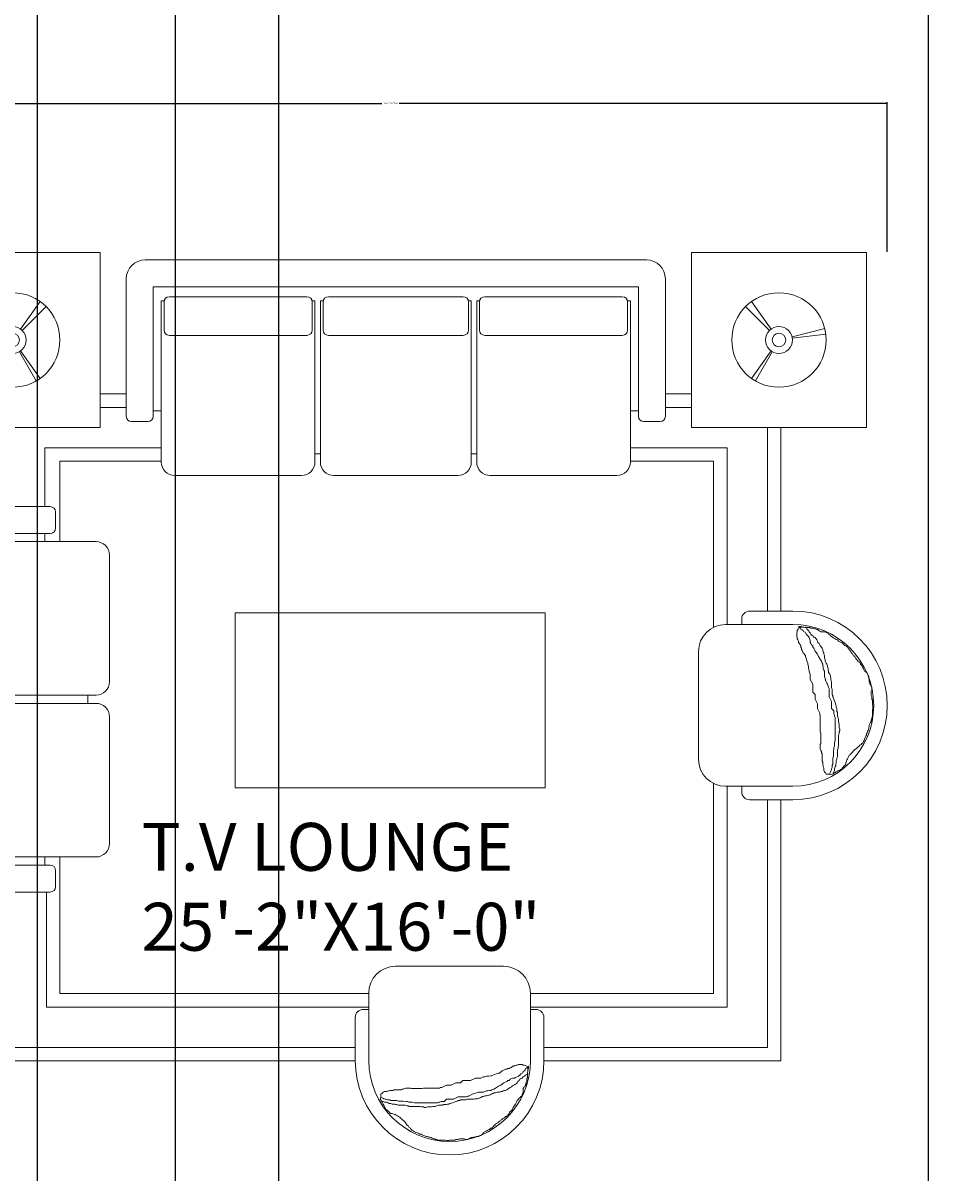
# Model space of a CAD drawing. Units: inches. Extents: x 2447 to 3157, y 2799 to 3988.
# Tile 6 of 9: x 2810 to 2947, y 3441 to 3609. Entities that reach past the tile are written whole.
import ezdxf

# ---------------------------------------------------------------- set-up
doc = ezdxf.new("R2010")
doc.units = ezdxf.units.IN
for name, color, linetype, lineweight in [('A-ANNO-DIMS', 2, 'Continuous', 18), ('A-AREA-IDEN', 7, 'Continuous', 25), ('A-FURN', 8, 'Continuous', 18)]:
    doc.layers.add(name, color=color, linetype=linetype, lineweight=lineweight)
doc.styles.get("Standard").update_dxf_attribs({"font": 'arial.ttf'})
doc.dimstyles.get("Standard").update_dxf_attribs({"dimtxt": 0.18, "dimasz": 0.18, "dimexe": 0.18, "dimexo": 0.0625, "dimgap": 0.09, "dimtad": 0, "dimtih": 1, "dimtoh": 1, "dimdec": 4, "dimzin": 0, "dimdsep": 46, "dimtxsty": 'Standard', "dimcen": 0.09, "dimadec": 0, "dimazin": 0, "dimtfac": 1, "dimtdec": 4, "dimtofl": 0, "dimtmove": 0, "dimatfit": 3, "dimfxl": 1, "dimtolj": 1, "dimtzin": 0, "dimarcsym": 0})

# ---------------------------------------------------------------- blocks, each defined once
blk = doc.blocks.new('A$C78064EA7')
for p, q in [((932.1, 3320.6), (2792.1, 3320.6)), ((862.1, 2740.6), (862.1, 3250.6)), ((2862.1, 3250.6), (2862.1, 2740.6)), ((962.1, 3220.6), (962.1, 2740.6)), ((2762.1, 3220.6), (962.1, 3220.6)), ((2762.1, 2740.6), (2762.1, 3220.6)), ((469.8, 3064.3), (542.4, 3166)), ((992.1, 3168.5), (1002.1, 3168.5)), ((992.1, 2570.6), (992.1, 3168.5)), ((1002.1, 3060.6), (1002.1, 3164.3)), ((1022.1, 3184.3), (1532.1, 3184.3)), ((1551.6, 3168.5), (1562.1, 3168.5)), ((1552.1, 3060.6), (1552.1, 3164.3)), ((1562.1, 2570.6), (1562.1, 3168.5)), ((1582.1, 3168.5), (1592.5, 3168.5)), ((1582.1, 2570.6), (1582.1, 3168.5)), ((1592.1, 3060.6), (1592.1, 3164.3)), ((1612.1, 3184.3), (2112.1, 3184.3)), ((2131.6, 3168.5), (2142.1, 3168.5)), ((2132.1, 3060.6), (2132.1, 3164.3)), ((2142.1, 2570.6), (2142.1, 3168.5)), ((2162.1, 3168.5), (2172.5, 3168.5)), ((2162.1, 2570.6), (2162.1, 3168.5)), ((2172.1, 3060.6), (2172.1, 3164.3)), ((2192.1, 3184.3), (2702.1, 3184.3)), ((2721.6, 3168.5), (2732.1, 3168.5)), ((2722.1, 3060.6), (2722.1, 3164.3)), ((2732.1, 3168.5), (2732.1, 2570.6)), ((3254.4, 3064.3), (3181.7, 3166)), ((476.1, 3059), (564.4, 3147.3)), ((3248.1, 3059), (3159.7, 3147.3)), ((391.1, 3029.8), (267.1, 3045.3)), ((392.2, 3035.7), (270.9, 3066)), ((1022.1, 3040.6), (1532.1, 3040.6)), ((1612.1, 3040.6), (2112.1, 3040.6)), ((2192.1, 3040.6), (2702.1, 3040.6)), ((3331.9, 3035.7), (3453.2, 3066)), ((3333, 3029.8), (3457.1, 3045.3)), ((465.5, 2980.2), (527.5, 2871.7)), ((469.8, 2982.9), (542.4, 2881.2)), ((3254.4, 2982.9), (3181.7, 2881.2)), ((3258.6, 2980.2), (3196.6, 2871.7)), ((862.1, 2823.6), (765.7, 2823.6)), ((2958.4, 2823.6), (2862.1, 2823.6)), ((862.1, 2773.6), (765.7, 2773.6)), ((2958.4, 2773.6), (2862.1, 2773.6)), ((962.1, 2760.6), (992.1, 2760.6)), ((2732.1, 2760.6), (2762.1, 2760.6)), ((365.7, 2698.6), (365.7, 2405.5)), ((415.7, 2698.6), (415.7, 2405.5)), ((942.1, 2720.6), (882.1, 2720.6)), ((2842.1, 2720.6), (2782.1, 2720.6)), ((3240.7, 2017.9), (3240.7, 2698.6)), ((3290.7, 2017.9), (3290.7, 2698.6)), ((992.1, 2623.6), (560, 2623.6)), ((560, 2405.5), (560, 2623.6)), ((992.1, 2573.6), (615.7, 2573.6)), ((615.7, 2573.6), (615.7, 2275.5)), ((1562.1, 2600.6), (1582.1, 2600.6)), ((2142.1, 2600.6), (2162.1, 2600.6)), ((1042.1, 2520.6), (1512.1, 2520.6)), ((1632.1, 2520.6), (2092.1, 2520.6)), ((2212.1, 2520.6), (2682.1, 2520.6)), ((70, 2405.5), (580, 2405.5)), ((600, 2385.5), (600, 2325.5)), ((0, 1045.5), (0, 2335.5)), ((580, 2305.5), (100, 2305.5)), ((100, 2305.5), (100, 1075.5)), ((560, 2275.5), (560, 2305.5)), ((152.1, 2275.5), (750, 2275.5)), ((152.1, 2265.1), (152.1, 2275.5)), ((260, 2265.5), (156.3, 2265.5)), ((136.3, 1735.5), (136.3, 2245.5)), ((280, 1735.5), (280, 2245.5)), ((800, 1755.5), (800, 2225.5)), ((3335.1, 2017.9), (3175.1, 2017.9)), ((3335.1, 1967.9), (3085.1, 1967.9)), ((3145.1, 1987.9), (3145.1, 1967.9)), ((3351.6, 1941.1), (3349.3, 1936.8)), ((3349.3, 1936.8), (3349.3, 1923.5)), ((3349.3, 1923.5), (3351.6, 1919.2)), ((3353.6, 1950), (3351.6, 1945.4)), ((3351.6, 1945.4), (3351.6, 1941.1)), ((3358.2, 1958.7), (3353.6, 1950)), ((3358.2, 1961), (3355.9, 1961)), ((3362.5, 1958.7), (3358.2, 1961)), ((3362.5, 1961), (3358.2, 1958.7)), ((3358.2, 1958.7), (3362.5, 1954.4)), ((3366.8, 1961), (3362.5, 1961)), ((3375.5, 1958.7), (3362.5, 1958.7)), ((3362.5, 1954.4), (3364.5, 1950)), ((3364.5, 1950), (3369.1, 1947.7)), ((3369.1, 1947.7), (3373.5, 1945.4)), ((3373.5, 1945.4), (3375.5, 1941.1)), ((3380.1, 1956.4), (3375.5, 1958.7)), ((3375.5, 1941.1), (3380.1, 1939.1)), ((3397.4, 1956.4), (3380.1, 1956.4)), ((3380.1, 1939.1), (3384.4, 1932.4)), ((3384.4, 1958.7), (3382.1, 1958.7)), ((3386.4, 1954.4), (3384.4, 1958.7)), ((3384.4, 1932.4), (3388.7, 1928.1)), ((3388.7, 1950), (3386.4, 1954.4)), ((3393.1, 1945.4), (3388.7, 1950)), ((3388.7, 1928.1), (3393.1, 1923.5)), ((3395.4, 1941.1), (3393.1, 1945.4)), ((3393.1, 1923.5), (3395.4, 1919.2)), ((3399.7, 1936.8), (3395.4, 1941.1)), ((3402, 1954.4), (3397.4, 1956.4)), ((3402, 1932.4), (3399.7, 1936.8)), ((3410.6, 1954.4), (3402, 1954.4)), ((3404, 1928.1), (3402, 1932.4)), ((3408.6, 1925.8), (3404, 1928.1)), ((3412.9, 1921.5), (3408.6, 1925.8)), ((3415, 1952.1), (3410.6, 1954.4)), ((3417.3, 1919.2), (3412.9, 1921.5)), ((3419.6, 1952.1), (3415, 1952.1)), ((3423.9, 1950), (3419.6, 1952.1)), ((3428.2, 1950), (3423.9, 1950)), ((3430.5, 1945.4), (3428.2, 1950)), ((3434.8, 1943.4), (3430.5, 1945.4)), ((3439.2, 1941.1), (3434.8, 1943.4)), ((3452.4, 1941.1), (3439.2, 1941.1)), ((3456.7, 1939.1), (3452.4, 1941.1)), ((3461.1, 1936.8), (3456.7, 1939.1)), ((3465.4, 1936.8), (3461.1, 1936.8)), ((3467.7, 1932.4), (3465.4, 1936.8)), ((3472, 1930.1), (3467.7, 1932.4)), ((3474.3, 1925.8), (3472, 1930.1)), ((3478.7, 1923.5), (3474.3, 1925.8)), ((3483, 1919.2), (3478.7, 1923.5)), ((3351.6, 1919.2), (3351.6, 1914.9)), ((3351.6, 1914.9), (3353.6, 1910.5)), ((3353.6, 1910.5), (3355.9, 1906.2)), ((3355.9, 1906.2), (3355.9, 1901.6)), ((3355.9, 1901.6), (3360.2, 1897.3)), ((3360.2, 1897.3), (3362.5, 1892.9)), ((3362.5, 1892.9), (3364.5, 1888.6)), ((3364.5, 1888.6), (3364.5, 1884.3)), ((3364.5, 1884.3), (3366.8, 1879.7)), ((3366.8, 1879.7), (3366.8, 1875.3)), ((3395.4, 1919.2), (3397.4, 1912.5)), ((3397.4, 1912.5), (3399.7, 1908.2)), ((3399.7, 1908.2), (3399.7, 1901.6)), ((3399.7, 1901.6), (3402, 1897.3)), ((3402, 1897.3), (3404, 1892.9)), ((3404, 1892.9), (3408.6, 1888.6)), ((3408.6, 1888.6), (3408.6, 1884.3)), ((3408.6, 1884.3), (3412.9, 1879.7)), ((3412.9, 1879.7), (3417.3, 1869)), ((3421.6, 1914.9), (3417.3, 1919.2)), ((3423.9, 1910.5), (3421.6, 1914.9)), ((3425.9, 1906.2), (3423.9, 1910.5)), ((3428.2, 1901.6), (3425.9, 1906.2)), ((3432.5, 1897.3), (3428.2, 1901.6)), ((3434.8, 1892.9), (3432.5, 1897.3)), ((3436.9, 1888.6), (3434.8, 1892.9)), ((3441.5, 1884.3), (3436.9, 1888.6)), ((3443.5, 1879.7), (3441.5, 1884.3)), ((3445.8, 1875.3), (3443.5, 1879.7)), ((3487.3, 1917.2), (3483, 1919.2)), ((3491.6, 1914.9), (3487.3, 1917.2)), ((3496.2, 1912.5), (3491.6, 1914.9)), ((3500.6, 1910.5), (3496.2, 1912.5)), ((3504.9, 1906.2), (3500.6, 1910.5)), ((3509.2, 1903.9), (3504.9, 1906.2)), ((3513.8, 1901.6), (3509.2, 1903.9)), ((3518.1, 1899.6), (3513.8, 1901.6)), ((3522.5, 1895.2), (3518.1, 1899.6)), ((3526.8, 1890.6), (3522.5, 1895.2)), ((3531.1, 1888.6), (3526.8, 1890.6)), ((3535.7, 1886.3), (3531.1, 1888.6)), ((3537.7, 1882), (3535.7, 1886.3)), ((3542.1, 1879.7), (3537.7, 1882)), ((3542.1, 1875.3), (3542.1, 1879.7)), ((2985.1, 1867.9), (2985.1, 1467.9)), ((3366.8, 1875.3), (3369.1, 1871)), ((3369.1, 1871), (3373.5, 1862.3)), ((3373.5, 1862.3), (3382.1, 1853.4)), ((3382.1, 1853.4), (3382.1, 1849.1)), ((3382.1, 1849.1), (3384.4, 1842.4)), ((3384.4, 1842.4), (3386.4, 1833.8)), ((3417.3, 1869), (3425.9, 1858)), ((3425.9, 1858), (3430.5, 1849.1)), ((3430.5, 1849.1), (3434.8, 1842.4)), ((3434.8, 1842.4), (3436.9, 1838.1)), ((3436.9, 1838.1), (3441.5, 1831.5)), ((3445.8, 1871), (3445.8, 1875.3)), ((3447.8, 1866.7), (3445.8, 1871)), ((3450.1, 1862.3), (3447.8, 1866.7)), ((3450.1, 1858), (3450.1, 1862.3)), ((3452.4, 1853.4), (3450.1, 1858)), ((3452.4, 1844.8), (3452.4, 1853.4)), ((3454.4, 1838.1), (3452.4, 1844.8)), ((3454.4, 1833.8), (3454.4, 1838.1)), ((3546.7, 1873.3), (3542.1, 1875.3)), ((3548.7, 1869), (3546.7, 1873.3)), ((3551, 1864.4), (3548.7, 1869)), ((3555.3, 1860), (3551, 1864.4)), ((3557.6, 1855.7), (3555.3, 1860)), ((3561.9, 1853.4), (3557.6, 1855.7)), ((3561.9, 1849.1), (3561.9, 1853.4)), ((3566.3, 1847.1), (3561.9, 1849.1)), ((3568.6, 1842.4), (3566.3, 1847.1)), ((3570.6, 1838.1), (3568.6, 1842.4)), ((3574.9, 1836.1), (3570.6, 1838.1)), ((3574.9, 1831.5), (3574.9, 1836.1)), ((3386.4, 1833.8), (3391, 1825.1)), ((3391, 1825.1), (3391, 1820.5)), ((3391, 1820.5), (3393.1, 1811.9)), ((3393.1, 1811.9), (3393.1, 1805.2)), ((3393.1, 1805.2), (3395.4, 1798.6)), ((3395.4, 1798.6), (3395.4, 1792.2)), ((3395.4, 1792.2), (3399.7, 1783.3)), ((3441.5, 1831.5), (3443.5, 1825.1)), ((3443.5, 1825.1), (3445.8, 1820.5)), ((3445.8, 1820.5), (3445.8, 1816.2)), ((3445.8, 1816.2), (3447.8, 1809.6)), ((3447.8, 1809.6), (3447.8, 1805.2)), ((3447.8, 1805.2), (3450.1, 1798.6)), ((3450.1, 1798.6), (3452.4, 1794.3)), ((3452.4, 1794.3), (3452.4, 1774.7)), ((3456.7, 1829.5), (3454.4, 1833.8)), ((3458.8, 1825.1), (3456.7, 1829.5)), ((3461.1, 1820.5), (3458.8, 1825.1)), ((3463.4, 1816.2), (3461.1, 1820.5)), ((3463.4, 1811.9), (3463.4, 1816.2)), ((3465.4, 1805.2), (3463.4, 1811.9)), ((3465.4, 1798.6), (3465.4, 1805.2)), ((3467.7, 1794.3), (3465.4, 1798.6)), ((3467.7, 1789.9), (3467.7, 1794.3)), ((3579.5, 1831.5), (3574.9, 1831.5)), ((3581.5, 1827.2), (3579.5, 1831.5)), ((3585.9, 1825.1), (3581.5, 1827.2)), ((3585.9, 1820.5), (3585.9, 1825.1)), ((3590.5, 1816.2), (3585.9, 1820.5)), ((3592.5, 1811.9), (3590.5, 1816.2)), ((3594.8, 1807.5), (3592.5, 1811.9)), ((3596.8, 1803.2), (3594.8, 1807.5)), ((3599.1, 1798.6), (3596.8, 1803.2)), ((3601.4, 1794.3), (3599.1, 1798.6)), ((3605.7, 1792.2), (3601.4, 1794.3)), ((3610.1, 1787.6), (3605.7, 1792.2)), ((3399.7, 1783.3), (3399.7, 1763.7)), ((3399.7, 1763.7), (3408.6, 1746.1)), ((3452.4, 1774.7), (3454.4, 1768)), ((3454.4, 1768), (3456.7, 1761.4)), ((3456.7, 1761.4), (3458.8, 1755)), ((3458.8, 1755), (3461.1, 1750.4)), ((3461.1, 1750.4), (3463.4, 1746.1)), ((3472, 1783.3), (3467.7, 1789.9)), ((3474.3, 1779), (3472, 1783.3)), ((3474.3, 1774.7), (3474.3, 1779)), ((3476.3, 1770.3), (3474.3, 1774.7)), ((3476.3, 1761.4), (3476.3, 1770.3)), ((3478.7, 1757.1), (3476.3, 1761.4)), ((3478.7, 1733.1), (3478.7, 1757.1)), ((3612.4, 1783.3), (3610.1, 1787.6)), ((3614.4, 1779), (3612.4, 1783.3)), ((3616.7, 1774.7), (3614.4, 1779)), ((3616.7, 1766), (3616.7, 1774.7)), ((3618.7, 1761.4), (3616.7, 1766)), ((3618.7, 1757.1), (3618.7, 1761.4)), ((3621, 1752.7), (3618.7, 1757.1)), ((3621, 1748.4), (3621, 1752.7)), ((152.1, 1705.5), (152.1, 1716)), ((260, 1715.5), (156.3, 1715.5)), ((3408.6, 1746.1), (3408.6, 1717.5)), ((3408.6, 1717.5), (3417.3, 1708.9)), ((3417.3, 1708.9), (3417.3, 1691.3)), ((3463.4, 1746.1), (3465.4, 1739.5)), ((3465.4, 1739.5), (3467.7, 1735.1)), ((3467.7, 1735.1), (3469.7, 1730.8)), ((3469.7, 1730.8), (3469.7, 1700.2)), ((3480.7, 1728.5), (3478.7, 1733.1)), ((3480.7, 1708.9), (3480.7, 1728.5)), ((3483, 1704.6), (3480.7, 1708.9)), ((3623.3, 1744.1), (3621, 1748.4)), ((3625.3, 1739.5), (3623.3, 1744.1)), ((3627.6, 1735.1), (3625.3, 1739.5)), ((3625.3, 1722.1), (3627.6, 1726.5)), ((3625.3, 1704.6), (3625.3, 1722.1)), ((3627.6, 1726.5), (3627.6, 1735.1)), ((750, 1705.5), (152.1, 1705.5)), ((750, 1675.5), (152.1, 1675.5)), ((152.1, 1665.1), (152.1, 1675.5)), ((260, 1665.5), (156.3, 1665.5)), ((720, 1685.5), (720, 1705.5)), ((720, 1675.5), (720, 1695.5)), ((3417.3, 1691.3), (3425.9, 1674)), ((3425.9, 1674), (3425.9, 1656.4)), ((3469.7, 1700.2), (3478.7, 1682.6)), ((3478.7, 1682.6), (3478.7, 1656.4)), ((3483, 1700.2), (3483, 1704.6)), ((3485.3, 1695.6), (3483, 1700.2)), ((3487.3, 1691.3), (3485.3, 1695.6)), ((3491.6, 1678.3), (3487.3, 1691.3)), ((3493.9, 1669.4), (3491.6, 1678.3)), ((3496.2, 1665), (3493.9, 1669.4)), ((3496.2, 1660.7), (3496.2, 1665)), ((3627.6, 1700.2), (3625.3, 1704.6)), ((3627.6, 1691.3), (3627.6, 1700.2)), ((3629.9, 1687), (3627.6, 1691.3)), ((3629.9, 1669.4), (3629.9, 1687)), ((3632, 1665), (3629.9, 1669.4)), ((3632, 1656.4), (3632, 1665)), ((136.3, 1135.5), (136.3, 1645.5)), ((280, 1135.5), (280, 1645.5)), ((800, 1155.5), (800, 1625.5)), ((3425.9, 1656.4), (3434.8, 1638.8)), ((3434.8, 1638.8), (3434.8, 1634.5)), ((3434.8, 1634.5), (3436.9, 1630.1)), ((3436.9, 1630.1), (3436.9, 1571)), ((3478.7, 1656.4), (3487.3, 1647.4)), ((3487.3, 1647.4), (3487.3, 1636.5)), ((3487.3, 1636.5), (3489.6, 1632.1)), ((3489.6, 1632.1), (3489.6, 1627.8)), ((3489.6, 1627.8), (3491.6, 1623.5)), ((3491.6, 1623.5), (3491.6, 1538.1)), ((3498.2, 1656.4), (3496.2, 1660.7)), ((3498.2, 1645.4), (3498.2, 1656.4)), ((3500.6, 1641.1), (3498.2, 1645.4)), ((3500.6, 1627.8), (3500.6, 1641.1)), ((3502.6, 1621.2), (3500.6, 1627.8)), ((3627.6, 1621.2), (3629.9, 1625.5)), ((3629.9, 1652), (3632, 1656.4)), ((3629.9, 1625.5), (3629.9, 1652)), ((3504.9, 1614.5), (3502.6, 1621.2)), ((3504.9, 1605.9), (3504.9, 1614.5)), ((3507.2, 1599.3), (3504.9, 1605.9)), ((3507.2, 1586.3), (3507.2, 1599.3)), ((3509.2, 1579.6), (3507.2, 1586.3)), ((3509.2, 1575.3), (3509.2, 1579.6)), ((3614.4, 1575.3), (3616.7, 1582)), ((3616.7, 1586.3), (3618.7, 1590.6)), ((3616.7, 1582), (3616.7, 1586.3)), ((3618.7, 1594.9), (3621, 1599.3)), ((3618.7, 1590.6), (3618.7, 1594.9)), ((3621, 1599.3), (3623.3, 1603.9)), ((3623.3, 1603.9), (3625.3, 1608.2)), ((3625.3, 1612.5), (3627.6, 1616.9)), ((3625.3, 1608.2), (3625.3, 1612.5)), ((3627.6, 1616.9), (3627.6, 1621.2)), ((3436.9, 1571), (3439.2, 1564.4)), ((3439.2, 1564.4), (3439.2, 1527.1)), ((3491.6, 1538.1), (3489.6, 1529.2)), ((3504.9, 1557.7), (3507.2, 1562)), ((3504.9, 1518.2), (3504.9, 1557.7)), ((3507.2, 1571), (3509.2, 1575.3)), ((3507.2, 1562), (3507.2, 1571)), ((3596.8, 1533.5), (3599.1, 1538.1)), ((3599.1, 1538.1), (3601.4, 1542.4)), ((3601.4, 1542.4), (3603.4, 1549.1)), ((3603.4, 1549.1), (3605.7, 1553.4)), ((3605.7, 1553.4), (3607.8, 1557.7)), ((3607.8, 1562), (3610.1, 1566.4)), ((3607.8, 1557.7), (3607.8, 1562)), ((3610.1, 1566.4), (3612.4, 1571)), ((3612.4, 1571), (3614.4, 1575.3)), ((3439.2, 1527.1), (3436.9, 1522.5)), ((3436.9, 1522.5), (3436.9, 1505.2)), ((3436.9, 1505.2), (3439.2, 1500.9)), ((3439.2, 1500.9), (3441.5, 1496.3)), ((3441.5, 1496.3), (3441.5, 1491.9)), ((3487.3, 1507.2), (3485.3, 1496.3)), ((3485.3, 1496.3), (3485.3, 1479)), ((3489.6, 1516.2), (3487.3, 1511.9)), ((3487.3, 1511.9), (3487.3, 1507.2)), ((3489.6, 1529.2), (3489.6, 1516.2)), ((3500.6, 1502.9), (3502.6, 1509.5)), ((3500.6, 1476.7), (3500.6, 1502.9)), ((3502.6, 1513.9), (3504.9, 1518.2)), ((3502.6, 1509.5), (3502.6, 1513.9)), ((3551, 1489.9), (3564, 1502.9)), ((3564, 1502.9), (3572.9, 1509.5)), ((3572.9, 1509.5), (3577.2, 1513.9)), ((3577.2, 1513.9), (3581.5, 1516.2)), ((3581.5, 1516.2), (3583.8, 1520.5)), ((3583.8, 1520.5), (3588.2, 1522.5)), ((3588.2, 1522.5), (3590.5, 1527.1)), ((3590.5, 1527.1), (3594.8, 1529.2)), ((3594.8, 1529.2), (3596.8, 1533.5)), ((3441.5, 1491.9), (3443.5, 1487.6)), ((3443.5, 1487.6), (3443.5, 1461.4)), ((3443.5, 1461.4), (3445.8, 1457)), ((3445.8, 1457), (3445.8, 1448.1)), ((3485.3, 1479), (3483, 1472.3)), ((3483, 1472.3), (3483, 1450.4)), ((3493.9, 1450.4), (3496.2, 1454.7)), ((3496.2, 1463.4), (3498.2, 1468)), ((3496.2, 1454.7), (3496.2, 1463.4)), ((3498.2, 1472.3), (3500.6, 1476.7)), ((3498.2, 1468), (3498.2, 1472.3)), ((3531.1, 1454.7), (3533.4, 1461.4)), ((3531.1, 1450.4), (3531.1, 1454.7)), ((3533.4, 1461.4), (3535.7, 1465.7)), ((3535.7, 1465.7), (3537.7, 1470)), ((3537.7, 1470), (3540, 1474.3)), ((3540, 1474.3), (3542.1, 1479)), ((3542.1, 1479), (3544.4, 1483.3)), ((3544.4, 1483.3), (3548.7, 1485.3)), ((3548.7, 1485.3), (3551, 1489.9)), ((3445.8, 1448.1), (3447.8, 1443.8)), ((3447.8, 1443.8), (3447.8, 1439.4)), ((3447.8, 1439.4), (3450.1, 1435.1)), ((3450.1, 1435.1), (3450.1, 1426.2)), ((3450.1, 1426.2), (3452.4, 1421.8)), ((3452.4, 1421.8), (3456.7, 1417.5)), ((3456.7, 1417.5), (3458.8, 1413.2)), ((3458.8, 1413.2), (3472, 1413.2)), ((3474.3, 1419.8), (3472, 1415.2)), ((3472, 1415.2), (3472, 1413.2)), ((3472, 1413.2), (3476.3, 1410.9)), ((3476.3, 1424.2), (3474.3, 1419.8)), ((3478.7, 1428.5), (3476.3, 1424.2)), ((3476.3, 1410.9), (3480.7, 1413.2)), ((3480.7, 1437.1), (3478.7, 1432.8)), ((3478.7, 1432.8), (3478.7, 1428.5)), ((3483, 1450.4), (3480.7, 1446.1)), ((3480.7, 1446.1), (3480.7, 1437.1)), ((3480.7, 1413.2), (3485.3, 1415.2)), ((3485.3, 1417.5), (3487.3, 1421.8)), ((3485.3, 1413.2), (3485.3, 1417.5)), ((3485.3, 1415.2), (3489.6, 1417.5)), ((3487.3, 1421.8), (3489.6, 1426.2)), ((3489.6, 1435.1), (3491.6, 1439.4)), ((3489.6, 1426.2), (3489.6, 1435.1)), ((3489.6, 1417.5), (3496.2, 1421.8)), ((3491.6, 1439.4), (3493.9, 1443.8)), ((3493.9, 1443.8), (3493.9, 1450.4)), ((3496.2, 1421.8), (3500.6, 1424.2)), ((3500.6, 1424.2), (3504.9, 1426.2)), ((3504.9, 1426.2), (3509.2, 1426.2)), ((3509.2, 1426.2), (3511.5, 1430.5)), ((3511.5, 1430.5), (3515.8, 1430.5)), ((3515.8, 1430.5), (3518.1, 1435.1)), ((3518.1, 1435.1), (3522.5, 1439.4)), ((3522.5, 1439.4), (3524.8, 1443.8)), ((3524.8, 1443.8), (3529.1, 1446.1)), ((3529.1, 1446.1), (3531.1, 1450.4)), ((3335.1, 1367.9), (3085.1, 1367.9)), ((3145.1, 1367.9), (3145.1, 1347.9)), ((3175.1, 1317.9), (3335.1, 1317.9)), ((152.1, 1105.5), (152.1, 1115.5)), ((260, 1115.5), (156.3, 1115.5)), ((100, 1075.5), (580, 1075.5)), ((750, 1105.5), (152.1, 1105.5)), ((560, 1075.5), (560, 1105.5)), ((600, 1055.5), (600, 995.5)), ((580, 975.5), (70, 975.5)), ((2261.5, 700), (1861.5, 700)), ((1761.5, 350), (1761.5, 600)), ((2361.5, 350), (2361.5, 600)), ((1761.5, 540), (1741.5, 540)), ((2381.5, 540), (2361.5, 540)), ((1711.5, 510), (1711.5, 350)), ((2411.5, 350), (2411.5, 510)), ((2236.1, 300.7), (2227.4, 298.6)), ((2242.7, 303), (2236.1, 300.7)), ((2247, 303), (2242.7, 303)), ((2256, 311.6), (2247, 303)), ((2264.6, 315.9), (2256, 311.6)), ((2269, 318.2), (2264.6, 315.9)), ((2273.3, 318.2), (2269, 318.2)), ((2277.9, 320.5), (2273.3, 318.2)), ((2282.2, 320.5), (2277.9, 320.5)), ((2286.6, 322.6), (2282.2, 320.5)), ((2290.9, 324.9), (2286.6, 322.6)), ((2295.2, 329.2), (2290.9, 324.9)), ((2299.8, 329.2), (2295.2, 329.2)), ((2304.2, 331.5), (2299.8, 329.2)), ((2308.5, 333.5), (2304.2, 331.5)), ((2312.8, 333.5), (2308.5, 333.5)), ((2317.1, 335.8), (2312.8, 333.5)), ((2330.4, 335.8), (2317.1, 335.8)), ((2326.1, 300.7), (2321.8, 296.3)), ((2332.7, 305), (2326.1, 300.7)), ((2334.7, 333.5), (2330.4, 335.8)), ((2334.7, 309.6), (2332.7, 305)), ((2339.1, 333.5), (2334.7, 333.5)), ((2339.1, 311.6), (2334.7, 309.6)), ((2343.7, 331.5), (2339.1, 333.5)), ((2341.4, 315.9), (2339.1, 311.6)), ((2343.7, 320.5), (2341.4, 315.9)), ((2352.3, 326.9), (2343.7, 331.5)), ((2348, 322.6), (2343.7, 320.5)), ((2352.3, 326.9), (2348, 322.6)), ((2348, 298.6), (2352.3, 300.7)), ((2350, 305), (2352.3, 309.6)), ((2350, 287.7), (2350, 305)), ((2352.3, 322.6), (2354.6, 326.9)), ((2354.6, 322.6), (2352.3, 326.9)), ((2352.3, 309.6), (2352.3, 322.6)), ((2352.3, 300.7), (2352.3, 303)), ((2354.6, 326.9), (2354.6, 329.2)), ((2354.6, 318.2), (2354.6, 322.6)), ((2050, 259.2), (2032.4, 250.2)), ((2067.6, 259.2), (2050, 259.2)), ((2084.9, 267.8), (2067.6, 259.2)), ((2102.5, 267.8), (2084.9, 267.8)), ((2111.2, 276.5), (2102.5, 267.8)), ((2139.7, 276.5), (2111.2, 276.5)), ((2157.3, 285.4), (2139.7, 276.5)), ((2176.9, 285.4), (2157.3, 285.4)), ((2185.9, 289.7), (2176.9, 285.4)), ((2192.2, 289.7), (2185.9, 289.7)), ((2198.9, 292), (2192.2, 289.7)), ((2205.5, 292), (2198.9, 292)), ((2214.2, 294), (2205.5, 292)), ((2218.8, 294), (2214.2, 294)), ((2227.4, 298.6), (2218.8, 294)), ((2251.7, 259.2), (2242.7, 254.6)), ((2262.6, 267.8), (2251.7, 259.2)), ((2273.3, 272.1), (2262.6, 267.8)), ((2277.9, 276.5), (2273.3, 272.1)), ((2282.2, 276.5), (2277.9, 276.5)), ((2286.6, 281.1), (2282.2, 276.5)), ((2290.9, 283.1), (2286.6, 281.1)), ((2295.2, 285.4), (2290.9, 283.1)), ((2290.9, 252.5), (2295.2, 256.9)), ((2301.9, 285.4), (2295.2, 285.4)), ((2295.2, 256.9), (2299.8, 259.2)), ((2299.8, 259.2), (2304.2, 261.2)), ((2306.2, 287.7), (2301.9, 285.4)), ((2304.2, 261.2), (2308.5, 263.5)), ((2312.8, 289.7), (2306.2, 287.7)), ((2308.5, 263.5), (2312.8, 267.8)), ((2317.1, 292), (2312.8, 289.7)), ((2312.8, 267.8), (2315.1, 272.1)), ((2315.1, 272.1), (2319.5, 276.5)), ((2321.8, 296.3), (2317.1, 292)), ((2319.5, 276.5), (2321.8, 281.1)), ((2321.8, 281.1), (2326.1, 283.1)), ((2326.1, 283.1), (2330.4, 285.4)), ((2330.4, 285.4), (2334.7, 289.7)), ((2334.7, 289.7), (2339.1, 292)), ((2339.1, 292), (2343.7, 296.3)), ((2339.1, 254.6), (2343.7, 256.9)), ((2343.7, 296.3), (2348, 298.6)), ((2343.7, 261.2), (2345.7, 265.5)), ((2343.7, 256.9), (2343.7, 261.2)), ((2345.7, 270.1), (2348, 274.4)), ((2345.7, 265.5), (2345.7, 270.1)), ((2348, 283.1), (2350, 287.7)), ((2348, 274.4), (2348, 283.1)), ((1811.2, 228.3), (1806.8, 226.3)), ((1806.8, 226.3), (1806.8, 213.1)), ((1815.5, 232.7), (1811.2, 228.3)), ((1819.8, 235), (1815.5, 232.7)), ((1828.8, 235), (1819.8, 235)), ((1833.1, 237.3), (1828.8, 235)), ((1837.4, 237.3), (1833.1, 237.3)), ((1841.7, 239.3), (1837.4, 237.3)), ((1850.7, 239.3), (1841.7, 239.3)), ((1855, 241.6), (1850.7, 239.3)), ((1881.3, 241.6), (1855, 241.6)), ((1885.6, 243.6), (1881.3, 241.6)), ((1889.9, 243.6), (1885.6, 243.6)), ((1894.5, 245.9), (1889.9, 243.6)), ((1898.9, 248.2), (1894.5, 245.9)), ((1916.2, 248.2), (1898.9, 248.2)), ((1920.8, 245.9), (1916.2, 248.2)), ((1958, 245.9), (1920.8, 245.9)), ((1964.6, 248.2), (1958, 245.9)), ((2023.8, 248.2), (1964.6, 248.2)), ((2028.1, 250.2), (2023.8, 248.2)), ((2032.4, 250.2), (2028.1, 250.2)), ((2093.9, 215.4), (2076.3, 206.4)), ((2124.4, 215.4), (2093.9, 215.4)), ((2128.8, 217.4), (2124.4, 215.4)), ((2133.1, 219.7), (2128.8, 217.4)), ((2139.7, 221.7), (2133.1, 219.7)), ((2144.1, 224), (2139.7, 221.7)), ((2148.7, 226.3), (2144.1, 224)), ((2155, 228.3), (2148.7, 226.3)), ((2161.7, 230.6), (2155, 228.3)), ((2168.3, 232.7), (2161.7, 230.6)), ((2187.9, 232.7), (2168.3, 232.7)), ((2176.9, 213.1), (2183.6, 217.4)), ((2183.6, 217.4), (2187.9, 217.4)), ((2192.2, 235), (2187.9, 232.7)), ((2187.9, 217.4), (2192.2, 219.7)), ((2198.9, 237.3), (2192.2, 235)), ((2192.2, 219.7), (2198.9, 219.7)), ((2203.2, 237.3), (2198.9, 237.3)), ((2198.9, 219.7), (2205.5, 221.7)), ((2209.8, 239.3), (2203.2, 237.3)), ((2205.5, 221.7), (2209.8, 221.7)), ((2214.2, 239.3), (2209.8, 239.3)), ((2209.8, 221.7), (2214.2, 224)), ((2218.8, 241.6), (2214.2, 239.3)), ((2214.2, 224), (2218.8, 226.3)), ((2225.1, 243.6), (2218.8, 241.6)), ((2218.8, 226.3), (2223.1, 228.3)), ((2223.1, 228.3), (2227.4, 230.6)), ((2231.8, 248.2), (2225.1, 243.6)), ((2227.4, 230.6), (2231.8, 230.6)), ((2236.1, 250.2), (2231.8, 248.2)), ((2231.8, 230.6), (2238.4, 232.7)), ((2242.7, 254.6), (2236.1, 250.2)), ((2238.4, 232.7), (2247, 232.7)), ((2247, 232.7), (2251.7, 235)), ((2251.7, 235), (2256, 235)), ((2256, 235), (2260.3, 237.3)), ((2260.3, 237.3), (2264.6, 239.3)), ((2264.6, 239.3), (2269, 239.3)), ((2269, 239.3), (2273.3, 241.6)), ((2273.3, 241.6), (2277.9, 243.6)), ((2277.9, 243.6), (2282.2, 248.2)), ((2282.2, 248.2), (2286.6, 250.2)), ((2286.6, 250.2), (2290.9, 252.5)), ((2323.8, 213.1), (2326.1, 217.4)), ((2326.1, 217.4), (2330.4, 219.7)), ((2330.4, 224), (2332.7, 228.3)), ((2330.4, 219.7), (2330.4, 224)), ((2332.7, 228.3), (2334.7, 232.7)), ((2334.7, 245.9), (2337.1, 250.2)), ((2334.7, 232.7), (2334.7, 245.9)), ((2337.1, 250.2), (2339.1, 254.6)), ((1806.8, 213.1), (1804.5, 208.7)), ((1804.5, 208.7), (1806.8, 204.4)), ((1808.9, 213.1), (1806.8, 213.1)), ((1806.8, 204.4), (1808.9, 199.8)), ((1806.8, 199.8), (1811.2, 199.8)), ((1813.5, 210.7), (1808.9, 213.1)), ((1808.9, 199.8), (1811.2, 195.5)), ((1811.2, 199.8), (1815.5, 197.8)), ((1811.2, 195.5), (1815.5, 188.8)), ((1817.8, 208.7), (1813.5, 210.7)), ((1815.5, 197.8), (1819.8, 195.5)), ((1815.5, 188.8), (1817.8, 184.5)), ((1822.1, 206.4), (1817.8, 208.7)), ((1817.8, 184.5), (1819.8, 180.2)), ((1819.8, 195.5), (1828.8, 195.5)), ((1819.8, 180.2), (1819.8, 175.9)), ((1819.8, 175.9), (1824.1, 173.6)), ((1826.5, 206.4), (1822.1, 206.4)), ((1824.1, 173.6), (1824.1, 169.2)), ((1830.8, 204.4), (1826.5, 206.4)), ((1828.8, 195.5), (1833.1, 193.5)), ((1839.7, 204.4), (1830.8, 204.4)), ((1833.1, 193.5), (1837.4, 191.2)), ((1837.4, 191.2), (1844, 191.2)), ((1844, 202.1), (1839.7, 204.4)), ((1866, 202.1), (1844, 202.1)), ((1844, 191.2), (1848.4, 188.8)), ((1848.4, 188.8), (1857, 188.8)), ((1857, 188.8), (1861.6, 186.8)), ((1861.6, 186.8), (1866, 186.8)), ((1872.6, 199.8), (1866, 202.1)), ((1866, 186.8), (1870.3, 184.5)), ((1870.3, 184.5), (1896.6, 184.5)), ((1889.9, 199.8), (1872.6, 199.8)), ((1900.9, 197.8), (1889.9, 199.8)), ((1896.6, 184.5), (1903.2, 182.5)), ((1905.5, 197.8), (1900.9, 197.8)), ((1903.2, 182.5), (1907.5, 182.5)), ((1909.8, 195.5), (1905.5, 197.8)), ((1907.5, 182.5), (1911.8, 180.2)), ((1922.8, 195.5), (1909.8, 195.5)), ((1911.8, 180.2), (1951.4, 180.2)), ((1931.7, 193.5), (1922.8, 195.5)), ((2017.1, 193.5), (1931.7, 193.5)), ((1951.4, 180.2), (1955.7, 177.9)), ((1955.7, 177.9), (1964.6, 177.9)), ((1964.6, 177.9), (1969, 175.9)), ((1969, 175.9), (1973.3, 175.9)), ((1973.3, 175.9), (1979.9, 177.9)), ((1979.9, 177.9), (1992.9, 177.9)), ((1992.9, 177.9), (1999.5, 180.2)), ((1999.5, 180.2), (2008.2, 180.2)), ((2008.2, 180.2), (2014.8, 182.5)), ((2014.8, 182.5), (2021.5, 184.5)), ((2021.5, 195.5), (2017.1, 193.5)), ((2025.8, 195.5), (2021.5, 195.5)), ((2021.5, 184.5), (2034.7, 184.5)), ((2030.1, 197.8), (2025.8, 195.5)), ((2041.1, 197.8), (2030.1, 197.8)), ((2034.7, 184.5), (2039.1, 186.8)), ((2039.1, 186.8), (2050, 186.8)), ((2050, 206.4), (2041.1, 197.8)), ((2076.3, 206.4), (2050, 206.4)), ((2050, 186.8), (2054.3, 188.8)), ((2054.3, 188.8), (2058.7, 188.8)), ((2058.7, 188.8), (2063, 191.2)), ((2063, 191.2), (2071.9, 193.5)), ((2071.9, 193.5), (2084.9, 197.8)), ((2084.9, 197.8), (2089.3, 199.8)), ((2089.3, 199.8), (2093.9, 202.1)), ((2093.9, 202.1), (2098.2, 202.1)), ((2098.2, 202.1), (2102.5, 204.4)), ((2102.5, 204.4), (2122.1, 204.4)), ((2122.1, 204.4), (2126.8, 206.4)), ((2126.8, 206.4), (2150.7, 206.4)), ((2150.7, 206.4), (2155, 208.7)), ((2155, 208.7), (2164, 208.7)), ((2164, 208.7), (2168.3, 210.7)), ((2168.3, 210.7), (2172.6, 210.7)), ((2172.6, 210.7), (2176.9, 213.1)), ((2293.2, 166.9), (2295.2, 171.3)), ((2295.2, 171.3), (2297.5, 175.9)), ((2297.5, 175.9), (2299.8, 180.2)), ((2299.8, 180.2), (2304.2, 184.5)), ((2304.2, 184.5), (2306.2, 188.8)), ((2306.2, 188.8), (2308.5, 193.5)), ((2308.5, 193.5), (2310.8, 197.8)), ((2310.8, 197.8), (2312.8, 202.1)), ((2312.8, 202.1), (2317.1, 206.4)), ((2317.1, 206.4), (2319.5, 210.7)), ((2319.5, 210.7), (2323.8, 213.1)), ((1824.1, 169.2), (1828.8, 166.9)), ((1828.8, 166.9), (1833.1, 162.6)), ((1833.1, 162.6), (1837.4, 160.3)), ((1837.4, 160.3), (1839.7, 156)), ((1839.7, 156), (1844, 154)), ((1844, 154), (1848.4, 154)), ((1848.4, 154), (1855, 151.7)), ((1855, 151.7), (1859.3, 149.4)), ((1859.3, 149.4), (1863.7, 147.3)), ((1863.7, 147.3), (1868, 145)), ((1868, 145), (1872.6, 143)), ((1872.6, 143), (1876.9, 140.7)), ((1876.9, 140.7), (1879, 136.4)), ((1879, 136.4), (1883.6, 134.1)), ((1883.6, 134.1), (1896.6, 121.1)), ((2249.4, 127.5), (2253.7, 129.8)), ((2253.7, 129.8), (2258, 134.1)), ((2258, 134.1), (2262.6, 136.4)), ((2262.6, 136.4), (2267, 138.4)), ((2267, 138.4), (2269, 143)), ((2269, 143), (2273.3, 143)), ((2273.3, 143), (2275.6, 147.3)), ((2275.6, 147.3), (2279.9, 149.4)), ((2279.9, 149.4), (2282.2, 154)), ((2282.2, 154), (2284.3, 158.3)), ((2284.3, 158.3), (2288.9, 162.6)), ((2288.9, 162.6), (2293.2, 166.9)), ((1896.6, 121.1), (1903.2, 112.2)), ((1903.2, 112.2), (1907.5, 107.9)), ((1907.5, 107.9), (1909.8, 103.5)), ((1909.8, 103.5), (1914.1, 101.2)), ((1914.1, 101.2), (1916.2, 96.9)), ((1916.2, 96.9), (1920.8, 94.6)), ((1920.8, 94.6), (1922.8, 90.3)), ((1922.8, 90.3), (1927.1, 88.3)), ((1927.1, 88.3), (1931.7, 86)), ((1931.7, 86), (1936.1, 83.7)), ((2187.9, 83.7), (2192.2, 86)), ((2192.2, 86), (2196.9, 88.3)), ((2196.9, 88.3), (2201.2, 90.3)), ((2201.2, 90.3), (2205.5, 92.6)), ((2205.5, 92.6), (2209.8, 94.6)), ((2209.8, 94.6), (2214.2, 99.2)), ((2214.2, 99.2), (2218.8, 99.2)), ((2218.8, 99.2), (2220.8, 103.5)), ((2220.8, 103.5), (2225.1, 105.6)), ((2225.1, 110.2), (2229.7, 110.2)), ((2225.1, 105.6), (2225.1, 110.2)), ((2229.7, 110.2), (2231.8, 114.5)), ((2231.8, 114.5), (2236.1, 116.5)), ((2236.1, 116.5), (2240.7, 118.8)), ((2240.7, 118.8), (2242.7, 123.1)), ((2242.7, 123.1), (2247, 123.1)), ((2247, 123.1), (2249.4, 127.5)), ((1936.1, 83.7), (1942.7, 81.6)), ((1942.7, 81.6), (1947, 79.3)), ((1947, 79.3), (1951.4, 77.3)), ((1951.4, 77.3), (1955.7, 77.3)), ((1955.7, 77.3), (1960, 75)), ((1960, 75), (1964.6, 72.7)), ((1964.6, 72.7), (1969, 70.7)), ((1969, 70.7), (1975.6, 68.4)), ((1975.6, 68.4), (1979.9, 68.4)), ((1979.9, 68.4), (1984.2, 66.4)), ((1984.2, 66.4), (1988.6, 66.4)), ((1988.6, 66.4), (1992.9, 64.1)), ((1992.9, 64.1), (1997.5, 61.8)), ((1997.5, 61.8), (2001.8, 59.7)), ((2001.8, 59.7), (2006.2, 59.7)), ((2006.2, 59.7), (2010.5, 57.4)), ((2010.5, 57.4), (2014.8, 57.4)), ((2014.8, 57.4), (2019.2, 55.1)), ((2019.2, 55.1), (2045.7, 55.1)), ((2045.7, 55.1), (2050, 53.1)), ((2050, 53.1), (2058.7, 53.1)), ((2058.7, 53.1), (2063, 55.1)), ((2063, 55.1), (2080.6, 55.1)), ((2080.6, 55.1), (2084.9, 57.4)), ((2084.9, 57.4), (2093.9, 57.4)), ((2093.9, 57.4), (2098.2, 59.7)), ((2098.2, 59.7), (2115.8, 59.7)), ((2115.8, 59.7), (2120.1, 57.4)), ((2120.1, 57.4), (2128.8, 57.4)), ((2128.8, 57.4), (2133.1, 59.7)), ((2133.1, 59.7), (2137.7, 61.8)), ((2137.7, 61.8), (2142, 64.1)), ((2142, 64.1), (2146.4, 64.1)), ((2146.4, 64.1), (2150.7, 66.4)), ((2150.7, 66.4), (2155, 66.4)), ((2155, 66.4), (2159.6, 68.4)), ((2159.6, 68.4), (2168.3, 68.4)), ((2168.3, 68.4), (2172.6, 70.7)), ((2172.6, 70.7), (2176.9, 72.7)), ((2176.9, 72.7), (2181.3, 75)), ((2181.3, 75), (2185.9, 79.3)), ((2185.9, 79.3), (2187.9, 83.7))]:
    blk.add_line(p, q)
for points in [[(765.7, 2698.6), (115.7, 2698.6), (115.7, 3348.6), (765.7, 3348.6)], [(2958.4, 2698.6), (3608.4, 2698.6), (3608.4, 3348.6), (2958.4, 3348.6)], [(1265.7, 1361.6), (1265.7, 2011.6), (2415.7, 2011.6), (2415.7, 1361.6)]]:
    blk.add_lwpolyline(points, close=True)
for points in [[(3090.7, 1967.9), (3090.7, 2623.6), (2732.1, 2623.6)], [(3040.7, 1957.5), (3040.7, 2573.6), (2732.1, 2573.6)], [(2361.5, 598.6), (3040.7, 598.6), (3040.7, 1378.2)], [(2361.5, 548.6), (3090.7, 548.6), (3090.7, 1367.9)], [(2411.5, 348.6), (3290.7, 348.6), (3290.7, 1317.9)], [(2411.5, 398.6), (3240.7, 398.6), (3240.7, 1317.9)], [(615.7, 1105.5), (615.7, 598.6), (1761.5, 598.6)], [(365.7, 975.5), (365.7, 348.6), (1711.5, 348.6)], [(415.7, 975.5), (415.7, 398.6), (1711.5, 398.6)], [(565.7, 975.5), (565.7, 548.6), (1761.5, 548.6)]]:
    blk.add_lwpolyline(points)
for centre, radius in [((440.7, 3023.6), 175), ((3283.4, 3023.6), 175), ((440.7, 3023.6), 50), ((3283.4, 3023.6), 50), ((440.7, 3023.6), 25), ((3283.4, 3023.6), 25)]:
    blk.add_circle(centre, radius)
for centre, radius, start, end in [((932.1, 3250.6), 70, 90, 180), ((2792.1, 3250.6), 70, 0, 90), ((1022.1, 3164.3), 20, 90, 180), ((1532.1, 3164.3), 20, 0, 90), ((1612.1, 3164.3), 20, 90, 180), ((2112.1, 3164.3), 20, 0, 90), ((2192.1, 3164.3), 20, 90, 180), ((2702.1, 3164.3), 20, 0, 90), ((1022.1, 3060.6), 20, 180, 270), ((1532.1, 3060.6), 20, 270, 0), ((1612.1, 3060.6), 20, 180, 270), ((2112.1, 3060.6), 20, 270, 0), ((2192.1, 3060.6), 20, 180, 270), ((2702.1, 3060.6), 20, 270, 0), ((882.1, 2740.6), 20, 180, 270), ((942.1, 2740.6), 20, 270, 0), ((2782.1, 2740.6), 20, 180, 270), ((2842.1, 2740.6), 20, 270, 0), ((1042.1, 2570.6), 50, 180, 270), ((1512.1, 2570.6), 50, 270, 0), ((1632.1, 2570.6), 50, 180, 270), ((2092.1, 2570.6), 50, 270, 0), ((2212.1, 2570.6), 50, 180, 270), ((2682.1, 2570.6), 50, 270, 0), ((70, 2335.5), 70, 90, 180), ((580, 2385.5), 20, 0, 90), ((580, 2325.5), 20, 270, 0), ((156.3, 2245.5), 20, 90, 180), ((260, 2245.5), 20, 0, 90), ((750, 2225.5), 50, 0, 90), ((3175.1, 1987.9), 30, 90, 180), ((3335.1, 1667.9), 350, 270, 90), ((3085.1, 1867.9), 100, 90, 180), ((3335.1, 1667.9), 300, 270, 90), ((750, 1755.5), 50, 270, 0), ((156.3, 1735.5), 20, 180, 270), ((260, 1735.5), 20, 270, 0), ((156.3, 1645.5), 20, 90, 180), ((260, 1645.5), 20, 0, 90), ((750, 1625.5), 50, 0, 90), ((3085.1, 1467.9), 100, 180, 270), ((3175.1, 1347.9), 30, 180, 270), ((750, 1155.5), 50, 270, 0), ((156.3, 1135.5), 20, 180, 270), ((260, 1135.5), 20, 270, 0), ((580, 1055.5), 20, 0, 90), ((70, 1045.5), 70, 180, 270), ((580, 995.5), 20, 270, 0), ((1861.5, 600), 100, 90, 180), ((2261.5, 600), 100, 0, 90), ((1741.5, 510), 30, 90, 180), ((2381.5, 510), 30, 0, 90), ((2061.5, 350), 350, 180, 0), ((2061.5, 350), 300, 180, 360)]:
    blk.add_arc(centre, radius, start, end)
blk = doc.blocks.new('*D34')
at = {"layer": 'A-ANNO-DIMS', "color": 0, "lineweight": -2, "transparency": 16777216}
for p, q in [((2791.4, 3575.51), (2791.4, 3597.39)), ((2791.58, 3597.21), (2862.68, 3597.21)), ((2936.3, 3597.21), (2865.19, 3597.21)), ((2936.48, 3575.51), (2936.48, 3597.39))]:
    blk.add_line(p, q, dxfattribs=at)
at = {"layer": 'A-ANNO-DIMS', "color": 0, "transparency": 16777216}
for points in [[(2791.58, 3597.24), (2791.58, 3597.18), (2791.4, 3597.21)], [(2936.3, 3597.24), (2936.3, 3597.18), (2936.48, 3597.21)]]:
    blk.add_solid(points, dxfattribs=at)
at = {"layer": 'Defpoints', "color": 0, "transparency": 16777216}
for p in [(2936.48, 3597.21), (2791.4, 3575.45), (2936.48, 3575.45)]:
    blk.add_point(p, dxfattribs=at)
at = {"layer": 'A-ANNO-DIMS', "color": 0, "transparency": 16777216, "insert": (2863.94, 3597.21), "char_height": 0.18, "attachment_point": 5}
blk.add_mtext('\\A1;LOUNGE SUITE 145', dxfattribs=at)
blk = doc.blocks.new('*D47')
at = {"layer": 'A-ANNO-DIMS', "color": 0, "lineweight": -2, "transparency": 16777216}
for p, q in [((2798.43, 3849.7), (3156.7, 3849.7)), ((3156.52, 3849.52), (3156.52, 3487.38)), ((3156.52, 3124.88), (3156.52, 3487.02)), ((3046.43, 3124.7), (3156.7, 3124.7))]:
    blk.add_line(p, q, dxfattribs=at)
at = {"layer": 'A-ANNO-DIMS', "color": 0, "transparency": 16777216}
for points in [[(3156.49, 3849.52), (3156.55, 3849.52), (3156.52, 3849.7)], [(3156.49, 3124.88), (3156.55, 3124.88), (3156.52, 3124.7)]]:
    blk.add_solid(points, dxfattribs=at)
at = {"layer": 'Defpoints', "color": 0, "transparency": 16777216}
for p in [(2798.37, 3849.7), (3156.52, 3849.7), (3046.37, 3124.7)]:
    blk.add_point(p, dxfattribs=at)
at = {"layer": 'A-ANNO-DIMS', "color": 0, "transparency": 16777216, "insert": (3156.52, 3487.2), "char_height": 0.18, "attachment_point": 5}
blk.add_mtext('\\A1;725', dxfattribs=at)
blk = doc.blocks.new('*D50')
at = {"layer": 'A-ANNO-DIMS', "color": 0, "lineweight": -2, "transparency": 16777216}
for p, q in [((2832.46, 3897.64), (2832.46, 2799.37)), ((2942.46, 3897.64), (2942.46, 2799.37)), ((2832.64, 2799.55), (2887.18, 2799.55)), ((2942.28, 2799.55), (2887.74, 2799.55))]:
    blk.add_line(p, q, dxfattribs=at)
at = {"layer": 'A-ANNO-DIMS', "color": 0, "transparency": 16777216}
for points in [[(2832.64, 2799.58), (2832.64, 2799.52), (2832.46, 2799.55)], [(2942.28, 2799.58), (2942.28, 2799.52), (2942.46, 2799.55)]]:
    blk.add_solid(points, dxfattribs=at)
at = {"layer": 'Defpoints', "color": 0, "transparency": 16777216}
for p in [(2832.46, 3897.7), (2942.46, 3897.7), (2942.46, 2799.55)]:
    blk.add_point(p, dxfattribs=at)
at = {"layer": 'A-ANNO-DIMS', "color": 0, "transparency": 16777216, "insert": (2887.46, 2799.55), "char_height": 0.18, "attachment_point": 5}
blk.add_mtext('\\A1;110', dxfattribs=at)
blk = doc.blocks.new('*D73')
at = {"layer": 'A-ANNO-DIMS', "color": 0, "lineweight": -2, "transparency": 16777216}
for p, q in [((2812.37, 3160.03), (2812.37, 3988.03)), ((2847.64, 3124.76), (2847.64, 3988.03)), ((2812.55, 3987.85), (2829.61, 3987.85)), ((2847.46, 3987.85), (2830.4, 3987.85))]:
    blk.add_line(p, q, dxfattribs=at)
at = {"layer": 'A-ANNO-DIMS', "color": 0, "transparency": 16777216}
for points in [[(2812.55, 3987.88), (2812.55, 3987.82), (2812.37, 3987.85)], [(2847.46, 3987.88), (2847.46, 3987.82), (2847.64, 3987.85)]]:
    blk.add_solid(points, dxfattribs=at)
at = {"layer": 'Defpoints', "color": 0, "transparency": 16777216}
for p in [(2847.64, 3987.85), (2812.37, 3159.97), (2847.64, 3124.7)]:
    blk.add_point(p, dxfattribs=at)
at = {"layer": 'A-ANNO-DIMS', "color": 0, "transparency": 16777216, "insert": (2830, 3987.85), "char_height": 0.18, "attachment_point": 5}
blk.add_mtext('\\A1;35.27', dxfattribs=at)
blk = doc.blocks.new('*D76')
at = {"layer": 'A-ANNO-DIMS', "color": 0, "lineweight": -2, "transparency": 16777216}
for p, q in [((2847.64, 3124.76), (2847.64, 3988.03)), ((2971.17, 3124.76), (2971.17, 3988.03)), ((2847.82, 3987.85), (2908.95, 3987.85)), ((2970.99, 3987.85), (2909.86, 3987.85))]:
    blk.add_line(p, q, dxfattribs=at)
at = {"layer": 'A-ANNO-DIMS', "color": 0, "transparency": 16777216}
for points in [[(2847.82, 3987.88), (2847.82, 3987.82), (2847.64, 3987.85)], [(2970.99, 3987.88), (2970.99, 3987.82), (2971.17, 3987.85)]]:
    blk.add_solid(points, dxfattribs=at)
at = {"layer": 'Defpoints', "color": 0, "transparency": 16777216}
for p in [(2971.17, 3987.85), (2847.64, 3124.7), (2971.17, 3124.7)]:
    blk.add_point(p, dxfattribs=at)
at = {"layer": 'A-ANNO-DIMS', "color": 0, "transparency": 16777216, "insert": (2909.4, 3987.85), "char_height": 0.18, "attachment_point": 5}
blk.add_mtext('\\A1;123.53', dxfattribs=at)

msp = doc.modelspace()

# ---------------------------------------------------------------- block references
at = {"layer": 'A-FURN', "xscale": 0.0393700787401575, "yscale": 0.0393700787401575, "zscale": 0.0393700787401575}
msp.add_blockref('A$C78064EA7', (2791.3965, 3443.6133), dxfattribs=at)

# ---------------------------------------------------------------- texts
at = {"layer": 'A-AREA-IDEN', "insert": (2827.5708, 3492.1122), "char_height": 7, "attachment_point": 1}
msp.add_mtext_dynamic_manual_height_columns('T.V LOUNGE\\P25\'-2"X16\'-0"', width=108.154933, gutter_width=12.5, heights=[0], dxfattribs=at)

# ---------------------------------------------------------------- dimensions: what is measured, and where the dimension line sits
at = {"layer": 'A-ANNO-DIMS'}
for base, p1, p2, override, picture, middle in [((2847.6393, 3987.8502), (2812.3672, 3159.9723), (2847.6393, 3124.7002), {"dimdec": 2, "dimlfac": 1, "dimrnd": 0, "dimzin": 0, "dimdsep": 46, "dimlunit": 2}, '*D73', (2830.0033, 3987.8502)), ((2971.1661, 3987.8502), (2847.6393, 3124.7002), (2971.1661, 3124.7002), {"dimdec": 2, "dimlfac": 1, "dimrnd": 0, "dimzin": 0, "dimdsep": 46, "dimlunit": 2}, '*D76', (2909.4027, 3987.8502)), ((2942.456, 2799.5502), (2832.456, 3897.7002), (2942.456, 3897.7002), {"dimdec": 0, "dimlfac": 1, "dimrnd": 0, "dimzin": 0, "dimdsep": 46, "dimlunit": 2}, '*D50', (2887.456, 2799.5502))]:
    dim = msp.add_linear_dim(base=base, p1=p1, p2=p2, dimstyle='Standard', override=override, dxfattribs=at)
    dim.commit()
    dim.dimension.update_dxf_attribs({"geometry": picture, "text_midpoint": middle})
dim = msp.add_linear_dim(base=(3156.5172, 3849.7002), p1=(3046.3672, 3124.7002), p2=(2798.3672, 3849.7002), angle=90, dimstyle='Standard', override={"dimdec": 0, "dimlfac": 1, "dimrnd": 0, "dimzin": 0, "dimdsep": 46, "dimlunit": 2}, dxfattribs=at)
dim.commit()
dim.dimension.update_dxf_attribs({"geometry": '*D47', "text_midpoint": (3156.5172, 3487.2002)})
dim = msp.add_linear_dim(base=(2936.4783, 3597.2104), p1=(2791.3965, 3575.4481), p2=(2936.4783, 3575.4481), text='LOUNGE SUITE <>', dimstyle='Standard', override={"dimdec": 0, "dimlfac": 1, "dimrnd": 0, "dimzin": 0, "dimdsep": 46, "dimlunit": 2}, dxfattribs=at)
dim.commit()
dim.dimension.update_dxf_attribs({"geometry": '*D34', "text_midpoint": (2863.9374, 3597.2104)})

doc.saveas('drawing.dxf')
